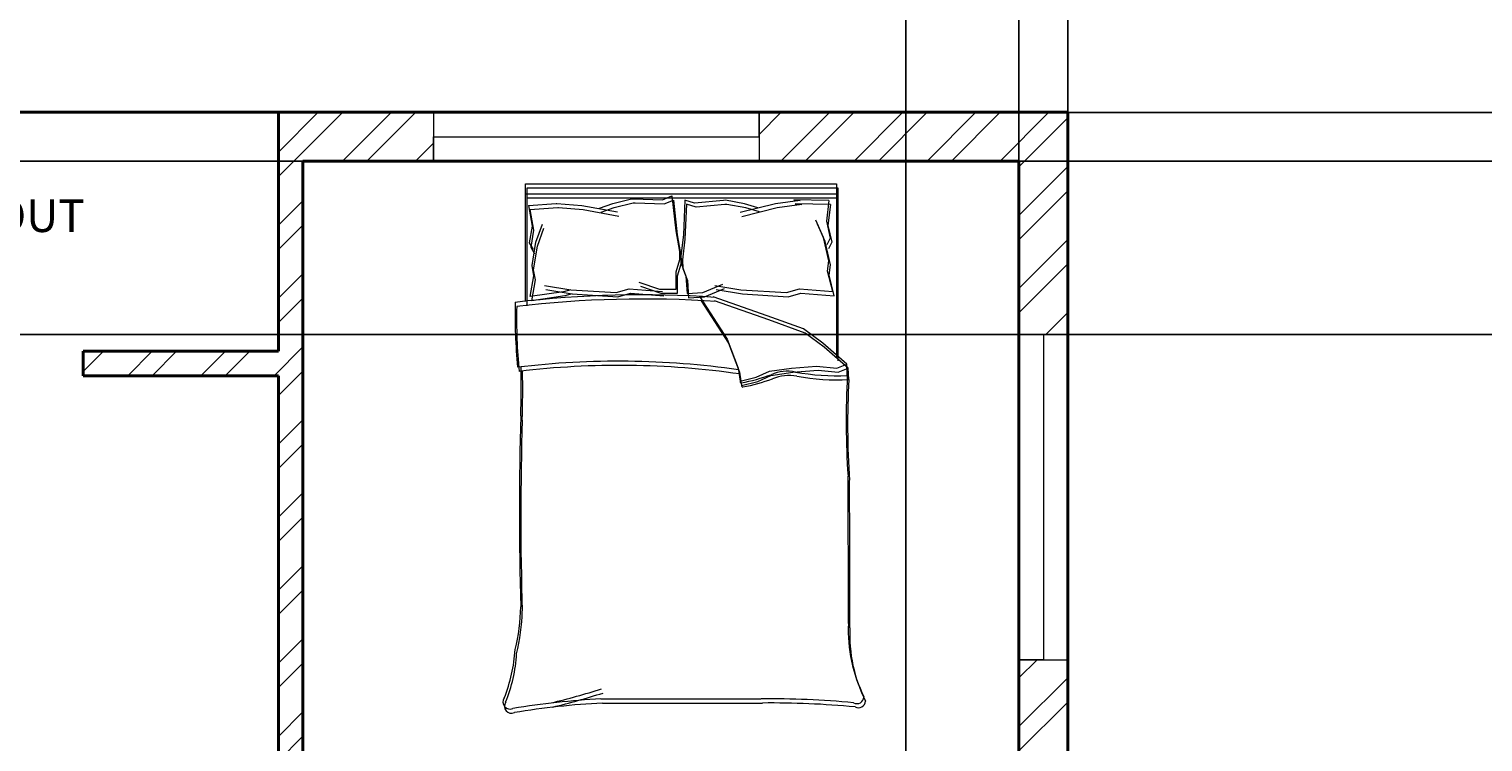
# Model space of a CAD drawing. Units: inches. Extents: x 1355 to 2746, y 1171 to 2751.
# Tile 13 of 24: x 1749 to 2017, y 2023 to 2155. Entities that reach past the tile are written whole.
import ezdxf

# ---------------------------------------------------------------- set-up
doc = ezdxf.new("R2010")
doc.units = ezdxf.units.IN
for name, color, linetype, lineweight in [('A-ANNO-DIMS', 2, 'Continuous', 18), ('A-AREA-IDEN', 7, 'Continuous', 18), ('A-FURN', 8, 'Continuous', 13), ('A-GLAZ', 4, 'Continuous', 18), ('A-WALL', 7, 'Continuous', 40), ('A-WALL-PATT', 252, 'Continuous', 13)]:
    doc.layers.add(name, color=color, linetype=linetype, lineweight=lineweight)
doc.styles.get("Standard").update_dxf_attribs({"font": 'arial.ttf'})
doc.dimstyles.get("Standard").update_dxf_attribs({"dimtxt": 0.18, "dimasz": 0.18, "dimexe": 0.18, "dimexo": 0.0625, "dimgap": 0.09, "dimtad": 0, "dimtih": 1, "dimtoh": 1, "dimdec": 4, "dimzin": 0, "dimdsep": 46, "dimtxsty": 'Standard', "dimcen": 0.09, "dimadec": 0, "dimazin": 0, "dimtfac": 1, "dimtdec": 4, "dimtofl": 0, "dimtmove": 0, "dimatfit": 3, "dimfxl": 1, "dimtolj": 1, "dimtzin": 0, "dimarcsym": 0})

# ---------------------------------------------------------------- blocks, each defined once
blk = doc.blocks.new('BED-DOUBLE-PLAN')
for p, q in [((75.16, 62.38), (96.87, 62.38)), ((75.93, 62.66), (97.64, 62.66)), ((77.72, 55.7), (76.85, 61.81)), ((76.85, 61.81), (80.66, 61.11)), ((85.96, 61.71), (84.75, 61.01)), ((86.73, 61.98), (85.52, 61.29)), ((89.08, 61.19), (85.96, 61.71)), ((89.85, 61.46), (86.73, 61.98)), ((92.9, 61.88), (89.08, 61.19)), ((93.66, 62.15), (89.85, 61.46)), ((92.87, 61.87), (93.27, 56.74)), ((93.64, 62.15), (94.03, 57.02)), ((95.03, 62.38), (95.03, 5.09)), ((95.8, 62.66), (95.8, 5.36)), ((96.87, 62.38), (96.87, 5.09)), ((97.64, 62.66), (97.64, 5.36)), ((76.95, 55.42), (76.08, 61.53)), ((76.08, 61.53), (79.9, 60.84)), ((78.9, 59.17), (78.1, 54.34)), ((79.9, 60.84), (81.8, 61.19)), ((80.66, 61.11), (82.57, 61.46)), ((81.8, 61.19), (86.14, 60.49)), ((82.57, 61.46), (86.9, 60.77)), ((86.14, 60.49), (89.43, 59.28)), ((86.9, 60.77), (90.2, 59.55)), ((78.14, 58.9), (77.34, 54.06)), ((93.24, 56.62), (92.9, 52.03)), ((93.27, 56.74), (93.24, 56.62)), ((94.01, 56.89), (93.66, 52.31)), ((94.03, 57.02), (94.01, 56.89)), ((77.34, 54.06), (76.82, 45.66)), ((77.34, 54.06), (76.95, 55.42)), ((78.1, 54.34), (77.59, 45.93)), ((78.1, 54.34), (77.72, 55.7)), ((92.9, 52.03), (91.68, 45.45)), ((93.66, 52.31), (92.45, 45.72)), ((1.87, 48.49), (1.87, 18.98)), ((2.64, 48.76), (2.64, 19.26)), ((92.38, 48.74), (93.24, 46.31)), ((93.14, 49.01), (94.01, 46.59)), ((76.82, 45.66), (77.49, 43.31)), ((77.59, 45.93), (78.25, 43.58)), ((93.24, 46.31), (94.11, 42.85)), ((94.01, 46.59), (94.88, 43.12)), ((77.49, 43.31), (77, 37.16)), ((78.25, 43.58), (77.77, 37.43)), ((94.88, 43.12), (94.88, 42.74)), ((77.38, 37.65), (78.68, 41.42)), ((78.14, 37.93), (79.45, 41.7)), ((94.11, 42.46), (93.94, 37.13)), ((94.11, 42.85), (94.11, 42.46)), ((94.88, 42.74), (94.7, 37.41)), ((77.38, 34.71), (77.38, 37.65)), ((78.14, 34.98), (78.14, 37.93)), ((81.36, 34.98), (78.14, 34.98)), ((83.61, 34.29), (81.36, 34.98)), ((88.98, 34.98), (85.17, 34.29)), ((94.63, 35.4), (88.22, 34.71)), ((95.4, 35.67), (88.98, 34.98)), ((93.94, 37.13), (94.63, 35.4)), ((94.7, 37.41), (95.4, 35.67)), ((79.83, 32.82), (76.62, 32.62)), ((76.62, 32.62), (76.8, 29.68)), ((80.59, 34.71), (77.38, 34.71)), ((80.6, 33.1), (77.39, 32.9)), ((77.39, 32.9), (77.57, 29.96)), ((82.03, 33.66), (79.83, 32.82)), ((82.84, 34.01), (80.59, 34.71)), ((82.8, 33.93), (80.6, 33.1)), ((83.59, 33.75), (82.03, 33.66)), ((84.36, 34.03), (82.8, 33.93)), ((84.4, 34.01), (82.84, 34.01)), ((87.44, 33.3), (83.59, 33.75)), ((85.17, 34.29), (83.61, 34.29)), ((88.21, 33.57), (84.36, 34.03)), ((88.22, 34.71), (84.4, 34.01)), ((93.89, 33.01), (87.44, 33.3)), ((94.65, 33.28), (88.21, 33.57)), ((93.3, 31.24), (93.89, 33.01)), ((94.07, 31.51), (94.65, 33.28)), ((76.03, 30.27), (68.25, 25.25)), ((76.8, 30.55), (69.01, 25.52)), ((76.8, 29.68), (78.34, 26)), ((77.57, 29.96), (79.11, 26.28)), ((93.81, 25.93), (93.3, 31.24)), ((94.57, 26.2), (94.07, 31.51)), ((72.52, 17.82), (76.03, 27.82)), ((73.28, 18.1), (76.8, 28.09)), ((78.14, 27.51), (77.34, 22.68)), ((78.9, 27.78), (78.1, 22.95)), ((68.25, 25.25), (62.87, 23.21)), ((69.01, 25.52), (63.63, 23.48)), ((93.18, 22.03), (93.83, 25.54)), ((93.83, 25.54), (93.81, 25.93)), ((93.95, 22.3), (94.6, 25.82)), ((94.6, 25.82), (94.57, 26.2)), ((62.87, 23.21), (60.45, 22.84)), ((60.45, 22.84), (61.2, 19.86)), ((63.63, 23.48), (61.22, 23.11)), ((61.22, 23.11), (61.96, 20.14)), ((77.34, 22.68), (76.82, 14.27)), ((78.1, 22.95), (77.59, 14.54)), ((93.19, 16.3), (91.57, 22.8)), ((93.96, 16.57), (92.34, 23.07)), ((92.47, 19.55), (93.18, 22.03)), ((93.23, 19.83), (93.95, 22.3)), ((61.2, 19.86), (62.31, 17.45)), ((61.96, 20.14), (63.08, 17.72)), ((62.31, 17.45), (62.87, 13.37)), ((63.08, 17.72), (63.63, 13.64)), ((70.1, 11.14), (72.52, 17.82)), ((70.87, 11.41), (73.28, 18.1)), ((93.82, 11.75), (93.19, 16.3)), ((94.59, 12.02), (93.96, 16.57)), ((63.63, 13.64), (64, 9)), ((76.82, 14.27), (77.49, 11.92)), ((77.59, 14.54), (78.25, 12.19)), ((62.87, 13.37), (63.24, 8.72)), ((67.51, 7.61), (70.1, 11.14)), ((68.27, 7.88), (70.87, 11.41)), ((77.49, 11.92), (77, 5.77)), ((78.25, 12.19), (77.77, 6.04)), ((93.81, 6.47), (93.92, 12.95)), ((93.92, 12.95), (93.82, 11.75)), ((94.57, 6.75), (94.69, 13.22)), ((94.69, 13.22), (94.59, 12.02)), ((63.24, 8.72), (62.87, 5.01)), ((64, 9), (63.63, 5.28)), ((86.97, 7.43), (90.18, 8.85)), ((87.74, 7.71), (90.95, 9.12)), ((63.61, 3.17), (67.51, 7.61)), ((64.38, 3.44), (68.27, 7.88)), ((97.64, 5.36), (65.74, 5.36)), ((77, 5.77), (80.77, 6.7)), ((77.77, 6.04), (81.53, 6.97)), ((80.77, 6.7), (82.69, 6.47)), ((81.53, 6.97), (83.46, 6.75)), ((82.69, 6.47), (86.97, 7.43)), ((83.46, 6.75), (87.74, 7.71)), ((86.88, 6.21), (85.62, 6.83)), ((87.64, 6.49), (86.39, 7.1)), ((89.96, 6.93), (86.88, 6.21)), ((90.72, 7.2), (87.64, 6.49)), ((93.81, 6.47), (89.96, 6.93)), ((94.57, 6.75), (90.72, 7.2)), ((61.52, 3.07), (63.61, 3.17, 4.64)), ((62.28, 3.35), (64.38, 3.44, 4.64)), ((62.87, 5.01), (63.61, 3.17)), ((63.63, 5.28), (64.38, 3.44)), ((96.87, 5.09), (64.97, 5.09))]:
    blk.add_line(p, q)
for centre, radius, start, end in [((1.3, 65.24), 1.31, 56.1736, 203.4781), ((-143.9, 40.86), 145.97, 2.9958, 9.4091), ((2.07, 65.52), 1.31, 56.1736, 203.4781), ((-143.14, 41.13), 145.97, 2.9958, 9.4091), ((12.62, 92.52), 28.25, 247.9751, 266.652), ((13.39, 92.79), 28.25, 247.9751, 266.652), ((20.29, 99.07), 35.53, 256.0648, 268.9113), ((73.55, -35.27), 99.87, 88.7218, 95.604), ((-120.62, 41.22), 197.77, 356.0865, 6.7821), ((19.53, 98.8), 35.53, 256.0648, 268.9113), ((36.19, -514.68), 578.22, 88.22771, 91.71854), ((36.96, -514.41), 578.22, 88.22771, 91.71854), ((59.5, 267.13), 203.94, 268.4762, 271.0082), ((60.27, 267.4), 203.94, 268.4762, 271.0082), ((-90.53, 45.26), 154.68, 351.7845, 6.9006), ((72.78, -35.55), 99.87, 88.7218, 95.604), ((-89.76, 45.54), 154.68, 351.7845, 6.9006), ((-121.38, 40.94), 197.77, 356.0865, 6.7821), ((125.3, 87.2), 127.63, 193.3832, 197.7053), ((126.07, 87.47), 127.63, 193.3832, 197.7053), ((60.38, 22.63), 0.221, 70.2464, 181.1377), ((95.1, 29.2), 35.55, 190.6617, 199.8806), ((61.15, 22.9), 0.221, 70.2464, 181.1377), ((95.86, 29.47), 35.55, 190.6617, 199.8806), ((-157.62, 17.21), 159.5, 354.4998, 0.6351), ((-156.85, 17.49), 159.5, 354.4998, 0.6351), ((54.83, 14.11), 7.46, 348.6608, 23.7384), ((55.6, 14.38), 7.46, 348.6608, 23.7384), ((104.85, 5.01), 43.38, 169.8763, 182.5657), ((105.62, 5.29), 43.38, 169.8763, 182.5657), ((14.55, -24.75), 27.65, 87.4714, 116.4681), ((15.32, -24.48), 27.65, 87.4714, 116.4681), ((15.56, 5471.89), 5469.02, 270.00217, 270.28689), ((16.33, 5472.16), 5469.02, 270.00217, 270.28689), ((53.34, -151.96), 155.25, 86.9791, 93.8365), ((54.1, -151.69), 155.25, 86.9791, 93.8365), ((2.32, 1.32), 1.32, 152.6588, 266.02), ((3.08, 1.59), 1.32, 152.6588, 266.02)]:
    blk.add_arc(centre, radius, start, end)
blk = doc.blocks.new('WINDOW-PLAN-60')
for p, q in [((0, 60), (9, 60)), ((9, 60), (4.5, 60)), ((4.5, 60), (4.5, 0)), ((4.5, 0), (0, 0)), ((0, 0), (9, 0))]:
    blk.add_line(p, q)
blk = doc.blocks.new('*D95')
at = {"layer": 'A-ANNO-DIMS', "color": 0, "lineweight": -2, "transparency": 16777216}
for p, q in [((1514.71, 2139.36), (1514.71, 2716.58)), ((1514.89, 2716.4), (1727.42, 2716.4)), ((1940.53, 2716.4), (1728, 2716.4)), ((1940.71, 2139.36), (1940.71, 2716.58))]:
    blk.add_line(p, q, dxfattribs=at)
at = {"layer": 'A-ANNO-DIMS', "color": 0, "transparency": 16777216}
for points in [[(1514.89, 2716.43), (1514.89, 2716.37), (1514.71, 2716.4)], [(1940.53, 2716.43), (1940.53, 2716.37), (1940.71, 2716.4)]]:
    blk.add_solid(points, dxfattribs=at)
at = {"layer": 'Defpoints', "color": 0, "transparency": 16777216}
for p in [(1940.71, 2716.4), (1514.71, 2139.3), (1940.71, 2139.3)]:
    blk.add_point(p, dxfattribs=at)
at = {"layer": 'A-ANNO-DIMS', "color": 0, "transparency": 16777216, "insert": (1727.71, 2716.4), "char_height": 0.18, "attachment_point": 5}
blk.add_mtext('\\A1;426', dxfattribs=at)
blk = doc.blocks.new('*D105')
at = {"layer": 'A-ANNO-DIMS', "color": 0, "lineweight": -2, "transparency": 16777216}
for p, q in [((2080.33, 2139.3), (1407.53, 2139.3)), ((1407.71, 2139.12), (1407.71, 2062.98)), ((1407.71, 1986.48), (1407.71, 2062.62)), ((2089.33, 1986.3), (1407.53, 1986.3))]:
    blk.add_line(p, q, dxfattribs=at)
at = {"layer": 'A-ANNO-DIMS', "color": 0, "transparency": 16777216}
for points in [[(1407.68, 2139.12), (1407.74, 2139.12), (1407.71, 2139.3)], [(1407.68, 1986.48), (1407.74, 1986.48), (1407.71, 1986.3)]]:
    blk.add_solid(points, dxfattribs=at)
at = {"layer": 'Defpoints', "color": 0, "transparency": 16777216}
for p in [(1407.71, 2139.3), (2080.39, 2139.3), (2089.39, 1986.3)]:
    blk.add_point(p, dxfattribs=at)
at = {"layer": 'A-ANNO-DIMS', "color": 0, "transparency": 16777216, "insert": (1407.71, 2062.8), "char_height": 0.18, "attachment_point": 5}
blk.add_mtext('\\A1;153', dxfattribs=at)
blk = doc.blocks.new('*D111')
at = {"layer": 'A-ANNO-DIMS', "color": 0, "lineweight": -2, "transparency": 16777216}
for p, q in [((2497.33, 2130.3), (1407.53, 2130.3)), ((1407.71, 2130.12), (1407.71, 2114.5)), ((1407.71, 2098.51), (1407.71, 2114.14)), ((2497.33, 2098.33), (1407.53, 2098.33))]:
    blk.add_line(p, q, dxfattribs=at)
at = {"layer": 'A-ANNO-DIMS', "color": 0, "transparency": 16777216}
for points in [[(1407.68, 2130.12), (1407.74, 2130.12), (1407.71, 2130.3)], [(1407.68, 2098.51), (1407.74, 2098.51), (1407.71, 2098.33)]]:
    blk.add_solid(points, dxfattribs=at)
at = {"layer": 'Defpoints', "color": 0, "transparency": 16777216}
for p in [(1407.71, 2130.3), (2497.39, 2130.3), (2497.39, 2098.33)]:
    blk.add_point(p, dxfattribs=at)
at = {"layer": 'A-ANNO-DIMS', "color": 0, "transparency": 16777216, "insert": (1407.71, 2114.32), "char_height": 0.18, "attachment_point": 5}
blk.add_mtext('\\A1;31.97', dxfattribs=at)
blk = doc.blocks.new('*D145')
at = {"layer": 'A-ANNO-DIMS', "color": 0, "lineweight": -2, "transparency": 16777216}
for p, q in [((1910.88, 1399.86), (1910.88, 2716.58)), ((1911.06, 2716.4), (1920.83, 2716.4)), ((1931.53, 2716.4), (1921.76, 2716.4)), ((1931.71, 1399.86), (1931.71, 2716.58))]:
    blk.add_line(p, q, dxfattribs=at)
at = {"layer": 'A-ANNO-DIMS', "color": 0, "transparency": 16777216}
for points in [[(1911.06, 2716.43), (1911.06, 2716.37), (1910.88, 2716.4)], [(1931.53, 2716.43), (1931.53, 2716.37), (1931.71, 2716.4)]]:
    blk.add_solid(points, dxfattribs=at)
at = {"layer": 'Defpoints', "color": 0, "transparency": 16777216}
for p in [(1931.71, 2716.4), (1910.88, 1399.8), (1931.71, 1399.8)]:
    blk.add_point(p, dxfattribs=at)
at = {"layer": 'A-ANNO-DIMS', "color": 0, "transparency": 16777216, "insert": (1921.3, 2716.4), "char_height": 0.18, "attachment_point": 5}
blk.add_mtext('\\A1;20.824', dxfattribs=at)

msp = doc.modelspace()

# ---------------------------------------------------------------- hatches: boundary and pattern name
at = {"layer": 'A-WALL-PATT'}
h = msp.add_hatch(dxfattribs=at)
h.set_pattern_fill('ANSI32', color=256)
h.paths.add_polyline_path([(1660.2083, 2139.3018), (1614.5977, 2139.3018), (1614.5977, 2130.3018), (1655.7083, 2130.3018), (1655.7083, 1981.8018), (1660.2083, 1981.8018), (1660.2083, 2090.7225), (1692.5832, 2090.7225), (1692.5832, 2095.2225), (1660.2083, 2095.2225)])
h.paths.add_polyline_path([(1523.7083, 2130.3018), (1554.5977, 2130.3018), (1554.5977, 2134.8018), (1554.5977, 2139.3018), (1514.7083, 2139.3018), (1514.7083, 2071.8385), (1523.7083, 2071.8385)])
h.paths.add_polyline_path([(1940.7083, 2139.3018), (1883.7928, 2139.3018), (1883.7928, 2130.3018), (1931.7083, 2130.3018), (1931.7083, 2098.3333), (1940.7083, 2098.3333)])
h.paths.add_polyline_path([(1799.7083, 2130.3018), (1823.7928, 2130.3018), (1823.7928, 2134.8018), (1823.7928, 2139.3018), (1795.2083, 2139.3018), (1795.2083, 2130.3018), (1795.2083, 2095.2225), (1759.2134, 2095.2225), (1759.2134, 2090.7225), (1795.2083, 2090.7225), (1795.2083, 1981.8018), (1799.7083, 1981.8018), (1799.7083, 1986.3018)])
h.paths.add_polyline_path([(1940.7083, 2038.3333), (1931.7083, 2038.3333), (1931.7083, 1986.3018), (1832.7083, 1986.3018), (1832.7083, 1947.1338), (1837.2083, 1947.1338), (1837.2083, 1981.8018), (1931.7083, 1981.8018), (1931.7083, 1967.1939), (1940.7083, 1967.1939)])
h.paths.add_polyline_path([(1940.7083, 1943.1939), (1931.7083, 1943.1939), (1931.7083, 1921.8018), (1837.2083, 1921.8018), (1837.2083, 1926.0511), (1832.7083, 1926.0511), (1832.7083, 1917.3018), (1931.7083, 1917.3018), (1931.7083, 1908.3321), (1940.7083, 1908.3321)])
h.paths.add_polyline_path([(1940.7083, 1884.3321), (1931.7083, 1884.3321), (1931.7083, 1869.3018), (1899.4583, 1869.3018), (1899.4583, 1864.8018), (1931.7083, 1864.8018), (1931.7083, 1773.3018), (1786.5143, 1773.3018), (1786.5143, 1764.3018), (1844.7083, 1764.3018), (1844.7083, 1748.9343), (1853.7083, 1748.9343), (1853.7083, 1764.3018), (1931.7083, 1764.3018), (1931.7083, 1652.9424), (1940.7083, 1652.9424)])
h.paths.add_polyline_path([(1799.7083, 1864.8018), (1806.0522, 1864.8018), (1806.0522, 1867.0518), (1806.0522, 1869.3018), (1799.7083, 1869.3018), (1799.7083, 1917.3018), (1799.7083, 1921.8018), (1795.2083, 1921.8018), (1795.2083, 1773.3018), (1799.7083, 1773.3018)])
h.paths.add_polyline_path([(1872.8988, 1867.0518), (1872.8988, 1869.3018), (1867.2083, 1869.3018), (1867.2083, 1917.3018), (1862.7083, 1917.3018), (1862.7083, 1869.3018), (1836.9546, 1869.3018), (1836.9546, 1864.8018), (1862.7083, 1864.8018), (1872.8988, 1864.8018)])
h.paths.add_polyline_path([(1749.2197, 1773.3018), (1655.7083, 1773.3018), (1523.7083, 1773.3018), (1523.7083, 1828.4963), (1514.7083, 1828.4963), (1514.7083, 1753.9033), (1519.2083, 1753.9033), (1523.7083, 1753.9033), (1523.7083, 1764.3018), (1655.7083, 1764.3018), (1749.2197, 1764.3018), (1749.2197, 1768.8018)])
h.paths.add_polyline_path([(1660.2083, 1921.8018), (1655.7083, 1921.8018), (1655.7083, 1917.3018), (1655.7083, 1773.3018), (1660.2083, 1773.3018)])
h.paths.add_polyline_path([(1523.7083, 2011.8385), (1514.7083, 2011.8385), (1514.7083, 1973.114), (1519.2083, 1973.114), (1523.7083, 1973.114), (1523.7083, 1976.8227), (1523.7083, 1981.8018), (1618.2083, 1981.8018), (1618.2083, 1921.8018), (1553.707, 1921.8018), (1553.707, 1917.3018), (1622.7083, 1917.3018), (1622.7083, 1919.5518), (1622.7083, 1921.8018), (1622.7083, 1986.3018), (1523.7083, 1986.3018)])
h.paths.add_polyline_path([(1529.6686, 1919.5518), (1529.6686, 1921.8018), (1523.7083, 1921.8018), (1523.7083, 1949.114), (1514.7083, 1949.114), (1514.7083, 1888.4963), (1523.7083, 1888.4963), (1523.7083, 1917.3018), (1529.6686, 1917.3018)])
h.paths.add_polyline_path([(1538.9419, 1775.643), (1585.5504, 1775.643), (1585.5504, 1798.0318), (1538.9419, 1798.0318)], flags=25)
h.paths.add_polyline_path([(1696.7097, 1497.3356), (1769.5651, 1497.3356), (1769.5651, 1523.4559), (1696.7097, 1523.4559)], flags=9)
h.paths.add_polyline_path([(1629.1643, 1230.5133), (1877.0879, 1230.5133), (1877.0879, 1267.606), (1629.1643, 1267.606)], flags=9)
h.paths.add_polyline_path([(2533.4462, 2215.4033), (2579.9292, 2215.4033), (2579.9292, 2231.889), (2533.4462, 2231.889)], flags=9)
h.paths.add_polyline_path([(2540.822, 2515.6945), (2594.2245, 2515.6945), (2594.2245, 2545.5463), (2540.822, 2545.5463)], flags=9)
h.paths.add_polyline_path([(2535.9857, 2588.2819), (2582.4687, 2588.2819), (2582.4687, 2604.7675), (2535.9857, 2604.7675)], flags=9)
h.paths.add_polyline_path([(2537.1627, 2617.1172), (2649.1245, 2617.1172), (2649.1245, 2633.6029), (2537.1627, 2633.6029)], flags=9)
h.paths.add_polyline_path([(2218.0051, 2168.228), (2363.9573, 2168.228), (2363.9573, 2205.3208), (2218.0051, 2205.3208)], flags=9)
h.paths.add_polyline_path([(1650.2156, 2165.3631), (1800.3547, 2165.3631), (1800.3547, 2202.4559), (1650.2156, 2202.4559)], flags=9)
h.paths.add_polyline_path([(2553.9592, 1610.7663), (2588.4203, 1610.7663), (2588.4203, 1660.2233), (2553.9592, 1660.2233)], flags=9)
h.paths.add_polyline_path([(1549.0868, 1648.2033), (1595.6952, 1648.2033), (1595.6952, 1670.5921), (1549.0868, 1670.5921)], flags=9)
h.paths.add_polyline_path([(1546.9525, 1502.0931), (1583.3413, 1502.0931), (1583.3413, 1524.4819), (1546.9525, 1524.4819)], flags=9)
h.paths.add_polyline_path([(1540.7704, 1433.4431), (1587.3788, 1433.4431), (1587.3788, 1455.8319), (1540.7704, 1455.8319)], flags=9)
h.paths.add_polyline_path([(1683.6524, 1321.5269), (1760.6169, 1321.5269), (1760.6169, 1333.8911), (1683.6524, 1333.8911)], flags=9)
h.paths.add_polyline_path([(1832.0485, 1356.0874), (1873.0989, 1356.0874), (1873.0989, 1378.4762), (1832.0485, 1378.4762)], flags=9)
h.paths.add_polyline_path([(1877.9694, 1431.2138), (1926.3827, 1431.2138), (1926.3827, 1453.578), (1877.9694, 1453.578)], flags=9)
h.paths.add_polyline_path([(1847.3106, 1499.8371), (1883.6994, 1499.8371), (1883.6994, 1522.2259), (1847.3106, 1522.2259)], flags=9)
h.paths.add_polyline_path([(1813.7015, 1640.7287), (1860.3099, 1640.7287), (1860.3099, 1663.1175), (1813.7015, 1663.1175)], flags=9)
h.paths.add_polyline_path([(1876.2576, 1710.2471), (1912.9452, 1710.2471), (1912.9452, 1732.6359), (1876.2576, 1732.6359)], flags=25)
h.paths.add_polyline_path([(1695.9163, 1715.3064), (1736.9668, 1715.3064), (1736.9668, 1737.6952), (1695.9163, 1737.6952)], flags=9)
h.paths.add_polyline_path([(1881.8583, 1888.9094), (1930.2717, 1888.9094), (1930.2717, 1911.2737), (1881.8583, 1911.2737)], flags=9)
h.paths.add_polyline_path([(1823.9298, 1798.6431), (1864.9803, 1798.6431), (1864.9803, 1821.0319), (1823.9298, 1821.0319)], flags=25)
h.paths.add_polyline_path([(1845.6062, 1948.1408), (1881.995, 1948.1408), (1881.995, 1970.5296), (1845.6062, 1970.5296)], flags=25)
h.paths.add_polyline_path([(1849.027, 1991.5151), (1895.6355, 1991.5151), (1895.6355, 2013.9039), (1849.027, 2013.9039)], flags=25)
h.paths.add_polyline_path([(1684.9725, 2113.8416), (1764.2658, 2113.8416), (1764.2658, 2126.2058), (1684.9725, 2126.2058)], flags=9)
h.paths.add_polyline_path([(1688.6193, 1913.0676), (1776.2005, 1913.0676), (1776.2005, 1935.4564), (1688.6193, 1935.4564)], flags=9)
h.paths.add_polyline_path([(1571.4689, 1930.9816), (1607.8577, 1930.9816), (1607.8577, 1953.3704), (1571.4689, 1953.3704)], flags=25)
h.paths.add_polyline_path([(1535.3581, 1998.3125), (1581.9665, 1998.3125), (1581.9665, 2020.7014), (1535.3581, 2020.7014)], flags=9)
h = msp.add_hatch(dxfattribs=at)
h.set_pattern_fill('ANSI32', color=256)
h.paths.add_polyline_path([(1749.2197, 1686.3018), (1732.6892, 1686.3018), (1523.7083, 1686.3018), (1523.7083, 1705.9033), (1514.7083, 1705.9033), (1514.7083, 1647.8732), (1519.2083, 1647.8732), (1523.7083, 1647.8732), (1523.7083, 1677.3018), (1655.7083, 1677.3018), (1655.7083, 1528.8018), (1660.2083, 1528.8018), (1660.2083, 1677.3018), (1732.6892, 1677.3018), (1749.2197, 1677.3018)])
h.paths.add_polyline_path([(1931.7083, 1686.3018), (1853.7083, 1686.3018), (1853.7083, 1703.5696), (1844.7083, 1703.5696), (1844.7083, 1686.3018), (1788.0274, 1686.3018), (1788.0274, 1677.3018), (1795.2083, 1677.3018), (1795.2083, 1528.8018), (1799.7083, 1528.8018), (1799.7083, 1677.3018), (1844.7083, 1677.3018), (1931.7083, 1677.3018)])
h.paths.add_polyline_path([(1931.7083, 1533.3018), (1844.7083, 1533.3018), (1832.7083, 1533.3018), (1832.7083, 1531.0518), (1832.7083, 1528.8018), (1832.7083, 1495.7519), (1837.2083, 1495.7519), (1837.2083, 1528.8018), (1931.7083, 1528.8018)])
h.paths.add_polyline_path([(1940.7083, 1592.9424), (1931.7083, 1592.9424), (1931.7083, 1506.7845), (1940.7083, 1506.7845)])
h.paths.add_polyline_path([(1940.7083, 1482.7845), (1936.2083, 1482.7845), (1931.7083, 1482.7845), (1931.7083, 1320.3018), (1880.7083, 1320.3018), (1880.7083, 1311.3018), (1940.7083, 1311.3018)])
h.paths.add_polyline_path([(1931.7083, 1468.8018), (1844.7083, 1468.8018), (1837.2083, 1468.8018), (1837.2083, 1474.34), (1832.7083, 1474.34), (1832.7083, 1468.8018), (1832.7083, 1464.3018), (1844.7083, 1464.3018), (1931.7083, 1464.3018)])
h.paths.add_polyline_path([(1863.8571, 1464.3018), (1859.3571, 1464.3018), (1859.3571, 1404.1662), (1838.1542, 1404.1662), (1838.1542, 1399.8018), (1869.4185, 1399.8018), (1869.4185, 1402.0518), (1869.4185, 1404.3018), (1863.8571, 1404.3018)])
h.paths.add_polyline_path([(1799.7083, 1399.6662), (1805.4082, 1399.6662), (1805.4082, 1401.9162), (1805.4082, 1404.1662), (1799.7083, 1404.1662), (1799.7083, 1464.3018), (1799.7083, 1468.8018), (1795.2083, 1468.8018), (1795.2083, 1356.2098), (1761.2597, 1356.2098), (1761.2597, 1351.7098), (1795.2083, 1351.7098), (1795.2083, 1320.3018), (1795.2083, 1311.3018), (1844.7083, 1311.3018), (1844.7083, 1315.8018), (1844.7083, 1320.3018), (1799.7083, 1320.3018)])
h.paths.add_polyline_path([(1692.9218, 1356.2098), (1660.2083, 1356.2098), (1660.2083, 1430.786), (1657.9583, 1430.786), (1655.7083, 1430.786), (1655.7083, 1320.3018), (1611.934, 1320.3018), (1611.934, 1311.3018), (1660.2083, 1311.3018), (1660.2083, 1351.7098), (1692.9218, 1351.7098)])
h.paths.add_polyline_path([(1523.7083, 1372.653), (1514.7083, 1372.653), (1514.7083, 1311.3018), (1551.934, 1311.3018), (1551.934, 1315.8018), (1551.934, 1320.3018), (1523.7083, 1320.3018)])
h.paths.add_polyline_path([(1523.7083, 1490.9023), (1514.7083, 1490.9023), (1514.7083, 1432.653), (1519.2083, 1432.653), (1523.7083, 1432.653)])
h.paths.add_polyline_path([(1660.2083, 1468.8018), (1622.7083, 1468.8018), (1622.7083, 1473.1566), (1618.2083, 1473.1566), (1618.2083, 1468.8018), (1523.7083, 1468.8018), (1523.7083, 1464.3018), (1655.7083, 1464.3018), (1655.7083, 1460.5634), (1660.2083, 1460.5634)])
h.paths.add_polyline_path([(1523.7083, 1587.8732), (1514.7083, 1587.8732), (1514.7083, 1514.9023), (1519.2083, 1514.9023), (1523.7083, 1514.9023)])
h.paths.add_polyline_path([(1622.7083, 1533.3018), (1523.7083, 1533.3018), (1523.7083, 1528.8018), (1618.2083, 1528.8018), (1618.2083, 1494.4205), (1622.7083, 1494.4205), (1622.7083, 1528.8018)])
h.paths.add_polyline_path([(1696.7097, 1497.3356), (1769.5651, 1497.3356), (1769.5651, 1523.4559), (1696.7097, 1523.4559)], flags=9)
h.paths.add_polyline_path([(1629.1643, 1230.5133), (1877.0879, 1230.5133), (1877.0879, 1267.606), (1629.1643, 1267.606)], flags=9)
h.paths.add_polyline_path([(2533.4462, 2215.4033), (2579.9292, 2215.4033), (2579.9292, 2231.889), (2533.4462, 2231.889)], flags=9)
h.paths.add_polyline_path([(2540.822, 2515.6945), (2594.2245, 2515.6945), (2594.2245, 2545.5463), (2540.822, 2545.5463)], flags=9)
h.paths.add_polyline_path([(2535.9857, 2588.2819), (2582.4687, 2588.2819), (2582.4687, 2604.7675), (2535.9857, 2604.7675)], flags=9)
h.paths.add_polyline_path([(2537.1627, 2617.1172), (2649.1245, 2617.1172), (2649.1245, 2633.6029), (2537.1627, 2633.6029)], flags=9)
h.paths.add_polyline_path([(2218.0051, 2168.228), (2363.9573, 2168.228), (2363.9573, 2205.3208), (2218.0051, 2205.3208)], flags=9)
h.paths.add_polyline_path([(1650.2156, 2165.3631), (1800.3547, 2165.3631), (1800.3547, 2202.4559), (1650.2156, 2202.4559)], flags=9)
h.paths.add_polyline_path([(2553.9592, 1610.7663), (2588.4203, 1610.7663), (2588.4203, 1660.2233), (2553.9592, 1660.2233)], flags=9)
h.paths.add_polyline_path([(1549.0868, 1648.2033), (1595.6952, 1648.2033), (1595.6952, 1670.5921), (1549.0868, 1670.5921)], flags=25)
h.paths.add_polyline_path([(1546.9525, 1502.0931), (1583.3413, 1502.0931), (1583.3413, 1524.4819), (1546.9525, 1524.4819)], flags=25)
h.paths.add_polyline_path([(1540.7704, 1433.4431), (1587.3788, 1433.4431), (1587.3788, 1455.8319), (1540.7704, 1455.8319)], flags=9)
h.paths.add_polyline_path([(1683.6524, 1321.5269), (1760.6169, 1321.5269), (1760.6169, 1333.8911), (1683.6524, 1333.8911)], flags=9)
h.paths.add_polyline_path([(1832.0485, 1356.0874), (1873.0989, 1356.0874), (1873.0989, 1378.4762), (1832.0485, 1378.4762)], flags=9)
h.paths.add_polyline_path([(1877.9694, 1431.2138), (1926.3827, 1431.2138), (1926.3827, 1453.578), (1877.9694, 1453.578)], flags=9)
h.paths.add_polyline_path([(1847.3106, 1499.8371), (1883.6994, 1499.8371), (1883.6994, 1522.2259), (1847.3106, 1522.2259)], flags=25)
h.paths.add_polyline_path([(1813.7015, 1640.7287), (1860.3099, 1640.7287), (1860.3099, 1663.1175), (1813.7015, 1663.1175)], flags=25)
h.paths.add_polyline_path([(1876.2576, 1710.2471), (1912.9452, 1710.2471), (1912.9452, 1732.6359), (1876.2576, 1732.6359)], flags=9)
h.paths.add_polyline_path([(1695.9163, 1715.3064), (1736.9668, 1715.3064), (1736.9668, 1737.6952), (1695.9163, 1737.6952)], flags=9)
h.paths.add_polyline_path([(1881.8583, 1888.9094), (1930.2717, 1888.9094), (1930.2717, 1911.2737), (1881.8583, 1911.2737)], flags=9)
h.paths.add_polyline_path([(1823.9298, 1798.6431), (1864.9803, 1798.6431), (1864.9803, 1821.0319), (1823.9298, 1821.0319)], flags=9)
h.paths.add_polyline_path([(1845.6062, 1948.1408), (1881.995, 1948.1408), (1881.995, 1970.5296), (1845.6062, 1970.5296)], flags=9)
h.paths.add_polyline_path([(1849.027, 1991.5151), (1895.6355, 1991.5151), (1895.6355, 2013.9039), (1849.027, 2013.9039)], flags=9)
h.paths.add_polyline_path([(1684.9725, 2113.8416), (1764.2658, 2113.8416), (1764.2658, 2126.2058), (1684.9725, 2126.2058)], flags=9)
h.paths.add_polyline_path([(1688.6193, 1913.0676), (1776.2005, 1913.0676), (1776.2005, 1935.4564), (1688.6193, 1935.4564)], flags=9)
h.paths.add_polyline_path([(1538.9419, 1775.643), (1585.5504, 1775.643), (1585.5504, 1798.0318), (1538.9419, 1798.0318)], flags=9)
h.paths.add_polyline_path([(1571.4689, 1930.9816), (1607.8577, 1930.9816), (1607.8577, 1953.3704), (1571.4689, 1953.3704)], flags=9)
h.paths.add_polyline_path([(1535.3581, 1998.3125), (1581.9665, 1998.3125), (1581.9665, 2020.7014), (1535.3581, 2020.7014)], flags=9)

# ---------------------------------------------------------------- linework, layer by layer
at = {"layer": 'A-WALL'}
for p, q in [((1660.2083, 2139.3018), (1795.2083, 2139.3018)), ((1795.2083, 2130.3018), (1795.2083, 2139.3018)), ((1795.2083, 2139.3018), (1940.7083, 2139.3018)), ((1940.7083, 2139.3018), (1940.7083, 1311.3018)), ((1795.2083, 2130.3018), (1795.2083, 2095.2225)), ((1799.7083, 2130.3018), (1799.7083, 1986.3018)), ((1799.7083, 2130.3018), (1931.7083, 2130.3018)), ((1931.7083, 2130.3018), (1931.7083, 1986.3018)), ((1759.2134, 2095.2225), (1759.2134, 2090.7225)), ((1759.2134, 2095.2225), (1795.2083, 2095.2225)), ((1795.2083, 2090.7225), (1759.2134, 2090.7225)), ((1795.2083, 2090.7225), (1795.2083, 1981.8018))]:
    msp.add_line(p, q, dxfattribs=at)

# ---------------------------------------------------------------- block references
at = {"layer": 'A-FURN', "rotation": 90.00000000000003}
msp.add_blockref('BED-DOUBLE-PLAN', (1903.4123, 2028.4798), dxfattribs=at)
at = {"layer": 'A-GLAZ', "extrusion": (0, 0, -1), "zscale": -1, "rotation": 270}
msp.add_blockref('WINDOW-PLAN-60', (-1883.793, 2139.302), dxfattribs=at)
at = {"layer": 'A-GLAZ'}
msp.add_blockref('WINDOW-PLAN-60', (1931.708, 2038.333), dxfattribs=at)

# ---------------------------------------------------------------- texts
at = {"layer": 'A-AREA-IDEN', "insert": (1686.8204, 2123.2243), "char_height": 6, "attachment_point": 1}
msp.add_mtext_dynamic_manual_height_columns('5\'0" WIDE SIT- OUT', width=100.672075, gutter_width=12.5, heights=[0], dxfattribs=at)

# ---------------------------------------------------------------- dimensions: what is measured, and where the dimension line sits
at = {"layer": 'A-ANNO-DIMS'}
for base, p1, p2, override, picture, middle in [((1940.7083, 2716.3999), (1514.7083, 2139.3018), (1940.7083, 2139.3018), {"dimdec": 0, "dimlfac": 1, "dimrnd": 0, "dimzin": 0, "dimdsep": 46, "dimlunit": 2}, '*D95', (1727.7083, 2716.3999)), ((1931.7083, 2716.3999), (1910.8842, 1399.8018), (1931.7083, 1399.8018), {"dimdec": 3, "dimlfac": 1, "dimrnd": 0, "dimzin": 0, "dimdsep": 46, "dimlunit": 2}, '*D145', (1921.2962, 2716.3999))]:
    dim = msp.add_linear_dim(base=base, p1=p1, p2=p2, dimstyle='Standard', override=override, dxfattribs=at)
    dim.commit()
    dim.dimension.update_dxf_attribs({"geometry": picture, "text_midpoint": middle})
for base, p1, p2, override, picture, middle in [((1407.7083, 2139.3018), (2089.3909, 1986.3018), (2080.3909, 2139.3018), {"dimdec": 0, "dimlfac": 1, "dimrnd": 0, "dimzin": 0, "dimdsep": 46, "dimlunit": 2}, '*D105', (1407.7083, 2062.8018)), ((1407.7083, 2130.3018), (2497.3909, 2098.3333), (2497.3909, 2130.3018), {"dimdec": 2, "dimlfac": 1, "dimrnd": 0, "dimzin": 0, "dimdsep": 46, "dimlunit": 2}, '*D111', (1407.7083, 2114.3176))]:
    dim = msp.add_linear_dim(base=base, p1=p1, p2=p2, angle=90, dimstyle='Standard', override=override, dxfattribs=at)
    dim.commit()
    dim.dimension.update_dxf_attribs({"geometry": picture, "text_midpoint": middle})

doc.saveas('drawing.dxf')
